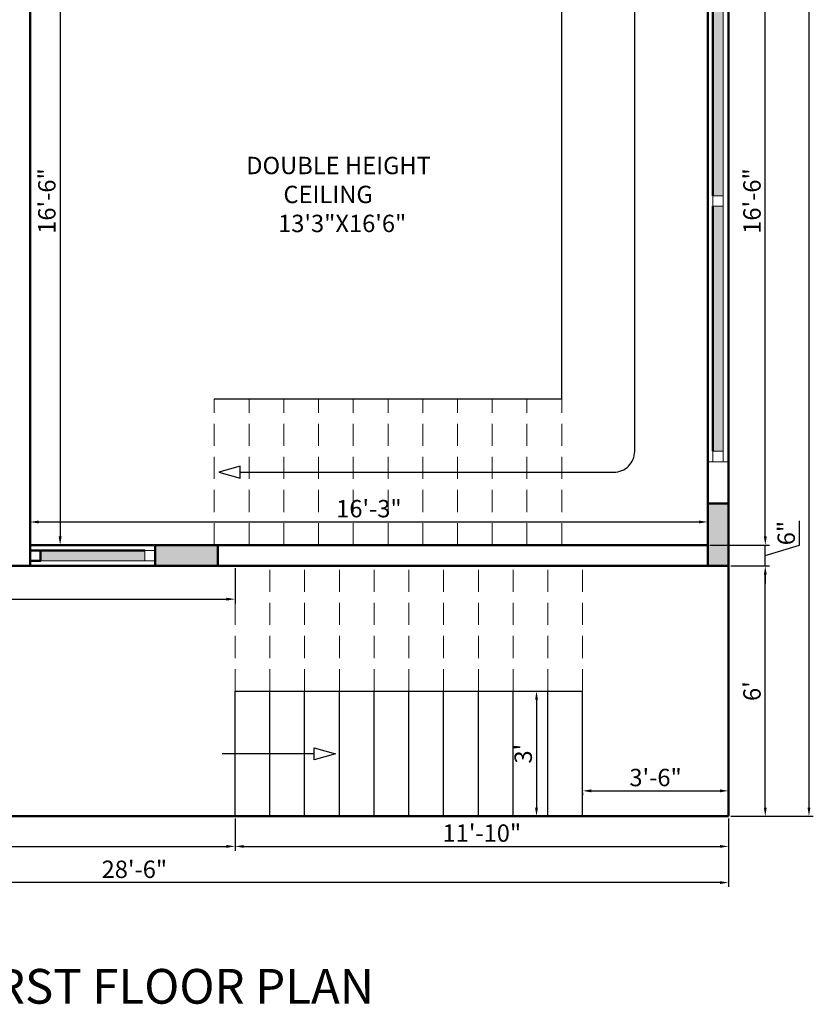
# Model space of a CAD drawing. Units: inches. Extents: x 3064 to 19385, y 846 to 15425.
# Tile 99 of 108: x 7664 to 7893, y 850 to 1134. Entities that reach past the tile are written whole.
import ezdxf

# ---------------------------------------------------------------- set-up
doc = ezdxf.new("R2010")
doc.units = ezdxf.units.IN
doc.linetypes.add('DASHED', pattern=[19.05, 12.7, -6.35])
for name, color, linetype, lineweight in [('A-ANNO-DIMS', 2, 'Continuous', 18), ('A-ANNO-TEXT', 7, 'Continuous', 25), ('A-AREA-IDEN', 3, 'Continuous', 18), ('A-COLS', 1, 'Continuous', 35), ('A-FLOR-STRS', 2, 'Continuous', 25), ('A-FLOR-STRS-OVHD', 2, 'DASHED', 18), ('A-GLAZ', 4, 'Continuous', 18), ('A-WALL', 7, 'Continuous', 50)]:
    doc.layers.add(name, color=color, linetype=linetype, lineweight=lineweight)
doc.styles.get("Standard").update_dxf_attribs({"font": 'arial.ttf'})
doc.dimstyles.new('ISO-25', dxfattribs={"dimtxt": 9, "dimasz": 2.5, "dimexe": 1.25, "dimexo": 0.625, "dimtad": 1, "dimdec": 1, "dimlunit": 3, "dimtxsty": 'Standard', "dimcen": 2.5, "dimadec": 0, "dimazin": 0, "dimtfac": 1, "dimtdec": 1, "dimtmove": 0, "dimatfit": 3, "dimfxl": 1, "dimarcsym": 0})

# ---------------------------------------------------------------- blocks, each defined once
blk = doc.blocks.new('*D325')
at = {"layer": 'A-ANNO-DIMS', "color": 0, "lineweight": -2, "transparency": 16777216}
for p, q in [((7526.25, 903.71), (7526.25, 894.42)), ((7726.25, 903.71), (7726.25, 894.42)), ((7528.75, 895.67), (7723.75, 895.67))]:
    blk.add_line(p, q, dxfattribs=at)
at = {"layer": 'A-ANNO-DIMS', "color": 0, "transparency": 16777216}
for points in [[(7528.75, 896.08), (7528.75, 895.25), (7526.25, 895.67)], [(7723.75, 896.08), (7723.75, 895.25), (7726.25, 895.67)]]:
    blk.add_solid(points, dxfattribs=at)
at = {"layer": 'Defpoints', "color": 0, "transparency": 16777216}
for p in [(7526.25, 904.34), (7726.25, 904.34), (7726.25, 895.67)]:
    blk.add_point(p, dxfattribs=at)
at = {"layer": 'A-ANNO-DIMS', "color": 0, "transparency": 16777216, "insert": (7626.25, 898.85), "char_height": 5, "attachment_point": 5}
blk.add_mtext('16\'-8"', dxfattribs=at)
blk = doc.blocks.new('*D326')
at = {"layer": 'A-ANNO-DIMS', "color": 0, "lineweight": -2, "transparency": 16777216}
for p, q in [((7726.25, 903.71), (7726.25, 894.42)), ((7868.25, 903.71), (7868.25, 894.42)), ((7728.75, 895.67), (7865.75, 895.67))]:
    blk.add_line(p, q, dxfattribs=at)
at = {"layer": 'A-ANNO-DIMS', "color": 0, "transparency": 16777216}
for points in [[(7728.75, 896.08), (7728.75, 895.25), (7726.25, 895.67)], [(7865.75, 896.08), (7865.75, 895.25), (7868.25, 895.67)]]:
    blk.add_solid(points, dxfattribs=at)
at = {"layer": 'Defpoints', "color": 0, "transparency": 16777216}
for p in [(7726.25, 904.34), (7868.25, 904.34), (7868.25, 895.67)]:
    blk.add_point(p, dxfattribs=at)
at = {"layer": 'A-ANNO-DIMS', "color": 0, "transparency": 16777216, "insert": (7797.25, 898.85), "char_height": 5, "attachment_point": 5}
blk.add_mtext('11\'-10"', dxfattribs=at)
blk = doc.blocks.new('*D224')
at = {"layer": 'A-ANNO-DIMS', "color": 0, "lineweight": -2, "transparency": 16777216}
for p, q in [((7526.25, 903.71), (7526.25, 884.01)), ((7868.25, 903.71), (7868.25, 884.01)), ((7865.75, 885.26), (7528.75, 885.26))]:
    blk.add_line(p, q, dxfattribs=at)
at = {"layer": 'A-ANNO-DIMS', "color": 0, "transparency": 16777216}
for points in [[(7528.75, 885.67), (7528.75, 884.84), (7526.25, 885.26)], [(7865.75, 885.67), (7865.75, 884.84), (7868.25, 885.26)]]:
    blk.add_solid(points, dxfattribs=at)
at = {"layer": 'Defpoints', "color": 0, "transparency": 16777216}
for p in [(7526.25, 904.34), (7868.25, 904.34), (7526.25, 885.26)]:
    blk.add_point(p, dxfattribs=at)
at = {"layer": 'A-ANNO-DIMS', "color": 0, "transparency": 16777216, "insert": (7697.25, 888.43), "char_height": 5, "attachment_point": 5}
blk.add_mtext('28\'-6"', dxfattribs=at)
blk = doc.blocks.new('*D327')
at = {"layer": 'A-ANNO-DIMS', "color": 0, "lineweight": -2, "transparency": 16777216}
for p, q in [((7868.87, 976.34), (7880.08, 976.34)), ((7878.83, 906.84), (7878.83, 973.84)), ((7868.87, 904.34), (7880.08, 904.34))]:
    blk.add_line(p, q, dxfattribs=at)
at = {"layer": 'A-ANNO-DIMS', "color": 0, "transparency": 16777216}
for points in [[(7878.41, 973.84), (7879.25, 973.84), (7878.83, 976.34)], [(7878.41, 906.84), (7879.25, 906.84), (7878.83, 904.34)]]:
    blk.add_solid(points, dxfattribs=at)
at = {"layer": 'Defpoints', "color": 0, "transparency": 16777216}
for p in [(7868.25, 976.34), (7878.83, 976.34), (7868.25, 904.34)]:
    blk.add_point(p, dxfattribs=at)
at = {"layer": 'A-ANNO-DIMS', "color": 0, "transparency": 16777216, "insert": (7875.65, 940.34), "char_height": 5, "attachment_point": 5, "rotation": 90}
blk.add_mtext("6'", dxfattribs=at)
blk = doc.blocks.new('*D328')
at = {"layer": 'A-ANNO-DIMS', "color": 0, "lineweight": -2, "transparency": 16777216}
for p, q in [((7888.67, 982.29), (7888.67, 989.32)), ((7878.83, 984.84), (7878.83, 987.34)), ((7862.87, 982.34), (7880.08, 982.34)), ((7878.83, 976.34), (7878.83, 982.34)), ((7878.83, 976.34), (7878.83, 982.34)), ((7878.83, 979.34), (7888.67, 982.29)), ((7868.87, 976.34), (7880.08, 976.34)), ((7878.83, 973.84), (7878.83, 971.34))]:
    blk.add_line(p, q, dxfattribs=at)
at = {"layer": 'A-ANNO-DIMS', "color": 0, "transparency": 16777216}
for points in [[(7878.41, 984.84), (7879.25, 984.84), (7878.83, 982.34)], [(7878.41, 973.84), (7879.25, 973.84), (7878.83, 976.34)]]:
    blk.add_solid(points, dxfattribs=at)
at = {"layer": 'Defpoints', "color": 0, "transparency": 16777216}
for p in [(7862.25, 982.34), (7878.83, 982.34), (7868.25, 976.34)]:
    blk.add_point(p, dxfattribs=at)
at = {"layer": 'A-ANNO-DIMS', "color": 0, "transparency": 16777216, "insert": (7885.5, 985.81), "char_height": 5, "attachment_point": 5, "rotation": 90}
blk.add_mtext('6"', dxfattribs=at)
blk = doc.blocks.new('*D329')
at = {"layer": 'A-ANNO-DIMS', "color": 0, "lineweight": -2, "transparency": 16777216}
for p, q in [((7868.87, 1180.34), (7880.08, 1180.34)), ((7878.83, 984.84), (7878.83, 1177.84)), ((7862.87, 982.34), (7880.08, 982.34))]:
    blk.add_line(p, q, dxfattribs=at)
at = {"layer": 'A-ANNO-DIMS', "color": 0, "transparency": 16777216}
for points in [[(7878.41, 1177.84), (7879.25, 1177.84), (7878.83, 1180.34)], [(7878.41, 984.84), (7879.25, 984.84), (7878.83, 982.34)]]:
    blk.add_solid(points, dxfattribs=at)
at = {"layer": 'Defpoints', "color": 0, "transparency": 16777216}
for p in [(7868.25, 1180.34), (7878.83, 1180.34), (7862.25, 982.34)]:
    blk.add_point(p, dxfattribs=at)
at = {"layer": 'A-ANNO-DIMS', "color": 0, "transparency": 16777216, "insert": (7875.65, 1081.34), "char_height": 5, "attachment_point": 5, "rotation": 90}
blk.add_mtext('16\'-6"', dxfattribs=at)
blk = doc.blocks.new('*D335')
at = {"layer": 'A-ANNO-DIMS', "color": 0, "lineweight": -2, "transparency": 16777216}
for p, q in [((7868.87, 1396.34), (7892.65, 1396.34)), ((7891.4, 1393.84), (7891.4, 906.84)), ((7868.87, 904.34), (7892.65, 904.34))]:
    blk.add_line(p, q, dxfattribs=at)
at = {"layer": 'A-ANNO-DIMS', "color": 0, "transparency": 16777216}
for points in [[(7890.98, 1393.84), (7891.82, 1393.84), (7891.4, 1396.34)], [(7890.98, 906.84), (7891.82, 906.84), (7891.4, 904.34)]]:
    blk.add_solid(points, dxfattribs=at)
at = {"layer": 'Defpoints', "color": 0, "transparency": 16777216}
for p in [(7868.25, 1396.34), (7868.25, 904.34), (7891.4, 904.34)]:
    blk.add_point(p, dxfattribs=at)
at = {"layer": 'A-ANNO-DIMS', "color": 0, "transparency": 16777216, "insert": (7888.27, 1150.34), "char_height": 5, "attachment_point": 5, "rotation": 90}
blk.add_mtext("41'", dxfattribs=at)
blk = doc.blocks.new('*D265')
at = {"layer": 'A-ANNO-DIMS', "color": 0, "lineweight": -2, "transparency": 16777216}
for p, q in [((7526.25, 975.71), (7526.25, 965.55)), ((7726.25, 975.71), (7726.25, 965.55)), ((7528.75, 966.8), (7723.75, 966.8))]:
    blk.add_line(p, q, dxfattribs=at)
at = {"layer": 'A-ANNO-DIMS', "color": 0, "transparency": 16777216}
for points in [[(7528.75, 967.22), (7528.75, 966.39), (7526.25, 966.8)], [(7723.75, 967.22), (7723.75, 966.39), (7726.25, 966.8)]]:
    blk.add_solid(points, dxfattribs=at)
at = {"layer": 'Defpoints', "color": 0, "transparency": 16777216}
for p in [(7526.25, 976.34), (7726.25, 976.34), (7726.25, 966.8)]:
    blk.add_point(p, dxfattribs=at)
at = {"layer": 'A-ANNO-DIMS', "color": 0, "transparency": 16777216, "insert": (7626.25, 969.98), "char_height": 5, "attachment_point": 5}
blk.add_mtext('16\'-8"', dxfattribs=at)
blk = doc.blocks.new('*D266')
at = {"layer": 'A-ANNO-DIMS', "color": 0, "lineweight": -2, "transparency": 16777216}
for p, q in [((7868.25, 912.28), (7868.25, 912.9)), ((7826.25, 911.03), (7826.25, 910.4)), ((7828.75, 911.65), (7865.75, 911.65))]:
    blk.add_line(p, q, dxfattribs=at)
at = {"layer": 'A-ANNO-DIMS', "color": 0, "transparency": 16777216}
for points in [[(7828.75, 912.07), (7828.75, 911.23), (7826.25, 911.65)], [(7865.75, 912.07), (7865.75, 911.23), (7868.25, 911.65)]]:
    blk.add_solid(points, dxfattribs=at)
at = {"layer": 'Defpoints', "color": 0, "transparency": 16777216}
for p in [(7826.25, 911.65), (7868.25, 911.65), (7868.25, 911.65)]:
    blk.add_point(p, dxfattribs=at)
at = {"layer": 'A-ANNO-DIMS', "color": 0, "transparency": 16777216, "insert": (7847.25, 914.83), "char_height": 5, "attachment_point": 5}
blk.add_mtext('3\'-6"', dxfattribs=at)
blk = doc.blocks.new('*D259')
at = {"layer": 'A-ANNO-DIMS', "color": 0, "lineweight": -2, "transparency": 16777216}
for p, q in [((7811.42, 940.34), (7814.24, 940.34)), ((7812.99, 937.84), (7812.99, 906.84)), ((7811.42, 904.34), (7814.24, 904.34))]:
    blk.add_line(p, q, dxfattribs=at)
at = {"layer": 'A-ANNO-DIMS', "color": 0, "transparency": 16777216}
for points in [[(7812.57, 937.84), (7813.41, 937.84), (7812.99, 940.34)], [(7812.57, 906.84), (7813.41, 906.84), (7812.99, 904.34)]]:
    blk.add_solid(points, dxfattribs=at)
at = {"layer": 'Defpoints', "color": 0, "transparency": 16777216}
for p in [(7810.8, 940.34), (7810.8, 904.34), (7812.99, 904.34)]:
    blk.add_point(p, dxfattribs=at)
at = {"layer": 'A-ANNO-DIMS', "color": 0, "transparency": 16777216, "insert": (7809.81, 922.34), "char_height": 5, "attachment_point": 5, "rotation": 90}
blk.add_mtext("3'", dxfattribs=at)
blk = doc.blocks.new('*D244')
at = {"layer": 'A-ANNO-DIMS', "color": 0, "lineweight": -2, "transparency": 16777216}
for p, q in [((7667.87, 1180.34), (7677.14, 1180.34)), ((7675.89, 1177.84), (7675.89, 984.84)), ((7667.87, 982.34), (7677.14, 982.34))]:
    blk.add_line(p, q, dxfattribs=at)
at = {"layer": 'A-ANNO-DIMS', "color": 0, "transparency": 16777216}
for points in [[(7675.47, 1177.84), (7676.3, 1177.84), (7675.89, 1180.34)], [(7675.47, 984.84), (7676.3, 984.84), (7675.89, 982.34)]]:
    blk.add_solid(points, dxfattribs=at)
at = {"layer": 'Defpoints', "color": 0, "transparency": 16777216}
for p in [(7667.25, 1180.34), (7667.25, 982.34), (7675.89, 982.34)]:
    blk.add_point(p, dxfattribs=at)
at = {"layer": 'A-ANNO-DIMS', "color": 0, "transparency": 16777216, "insert": (7672.71, 1081.34), "char_height": 5, "attachment_point": 5, "rotation": 90}
blk.add_mtext('16\'-6"', dxfattribs=at)
blk = doc.blocks.new('*D245')
at = {"layer": 'A-ANNO-DIMS', "color": 0, "lineweight": -2, "transparency": 16777216}
for p, q in [((7667.25, 982.96), (7667.25, 990.26)), ((7669.75, 989.01), (7859.75, 989.01)), ((7862.25, 982.96), (7862.25, 990.26))]:
    blk.add_line(p, q, dxfattribs=at)
at = {"layer": 'A-ANNO-DIMS', "color": 0, "transparency": 16777216}
for points in [[(7669.75, 989.43), (7669.75, 988.6), (7667.25, 989.01)], [(7859.75, 989.43), (7859.75, 988.6), (7862.25, 989.01)]]:
    blk.add_solid(points, dxfattribs=at)
at = {"layer": 'Defpoints', "color": 0, "transparency": 16777216}
for p in [(7862.25, 989.01), (7667.25, 982.34), (7862.25, 982.34)]:
    blk.add_point(p, dxfattribs=at)
at = {"layer": 'A-ANNO-DIMS', "color": 0, "transparency": 16777216, "insert": (7764.75, 992.19), "char_height": 5, "attachment_point": 5}
blk.add_mtext('16\'-3"', dxfattribs=at)
blk = doc.blocks.new('WIN-1800-PAIR')
h = blk.add_hatch(color=256)
h.dxf.hatch_style = 1
h.paths.add_polyline_path([(0, 0), (3, 0), (3, 70.5), (0, 70.5)])
h.paths.add_polyline_path([(3, 144), (0, 144), (0, 73.5), (3, 73.5)])
blk.add_line((3, 144), (3, 73.5))
blk.add_lwpolyline([(3, 144), (0, 144), (0, 147), (3, 147)], close=True)
blk = doc.blocks.new('WIN-900')
blk.add_line((0, 0), (30, 0))
blk.add_lwpolyline([(30, 0), (30, 3), (33, 3), (33, 0)], close=True)
blk = doc.blocks.new('WIN-2000')
blk.add_line((3, 0), (3, 70.5))
blk.add_lwpolyline([(3, 70.5), (0, 70.5), (0, 73.5), (3, 73.5)], close=True)

msp = doc.modelspace()

# ---------------------------------------------------------------- hatches: boundary and pattern name
at = {"layer": 'A-COLS'}
h = msp.add_hatch(color=256, dxfattribs=at)
h.dxf.hatch_style = 1
h.paths.add_polyline_path([(7862.25, 976.34), (7868.25, 976.34), (7868.25, 994.34), (7862.25, 994.34)])
h = msp.add_hatch(color=256, dxfattribs=at)
h.dxf.hatch_style = 1
h.paths.add_polyline_path([(7721.25, 976.34), (7721.25, 982.34), (7703.25, 982.34), (7703.25, 976.34)])
at = {"layer": 'A-GLAZ'}
h = msp.add_hatch(color=256, dxfattribs=at)
h.dxf.hatch_style = 1
h.paths.add_polyline_path([(7670.25, 980.84), (7670.25, 977.84), (7700.25, 977.84), (7700.25, 980.84)])

# ---------------------------------------------------------------- linework, layer by layer
at = {"layer": 'A-FLOR-STRS'}
for p, q in [((7820.25, 1024.34), (7820.25, 1180.34)), ((7820.25, 1024.34), (7720.25, 1024.34)), ((7726.25, 904.34), (7726.25, 940.34)), ((7726.25, 940.34), (7826.25, 940.34)), ((7736.25, 904.34), (7736.25, 940.34)), ((7746.25, 904.34), (7746.25, 940.34)), ((7756.25, 904.34), (7756.25, 940.34)), ((7766.25, 904.34), (7766.25, 940.34)), ((7776.25, 904.34), (7776.25, 940.34)), ((7786.25, 904.34), (7786.25, 940.34)), ((7796.25, 904.34), (7796.25, 940.34)), ((7806.25, 904.34), (7806.25, 940.34)), ((7816.25, 904.34), (7816.25, 940.34)), ((7826.25, 904.34), (7826.25, 940.34)), ((7748.95, 922.34), (7722.56, 922.34))]:
    msp.add_line(p, q, dxfattribs=at)
msp.add_lwpolyline([(7727.74, 1003.34), (7835.25, 1003.34, 0.414214), (7841.25, 1009.34), (7841.25, 1153.34, 0.414214), (7835.25, 1159.34), (7708.25, 1159.34)], format="xyb", dxfattribs=at)
for points in [[(7721.54, 1003.34), (7727.74, 1001.61), (7727.74, 1005.07)], [(7755.14, 922.34), (7748.95, 920.61), (7748.95, 924.07)]]:
    msp.add_lwpolyline(points, close=True, dxfattribs=at)
at = {"layer": 'A-FLOR-STRS-OVHD', "ltscale": 0.5}
for p, q in [((7720.25, 982.34), (7720.25, 1024.34)), ((7730.25, 982.34), (7730.25, 1024.34)), ((7740.25, 982.34), (7740.25, 1024.34)), ((7750.25, 982.34), (7750.25, 1024.34)), ((7760.25, 982.34), (7760.25, 1024.34)), ((7770.25, 982.34), (7770.25, 1024.34)), ((7780.25, 982.34), (7780.25, 1024.34)), ((7790.25, 982.34), (7790.25, 1024.34)), ((7800.25, 982.34), (7800.25, 1024.34)), ((7810.25, 982.34), (7810.25, 1024.34)), ((7820.25, 982.34), (7820.25, 1024.34)), ((7726.25, 940.34), (7726.25, 976.34)), ((7736.25, 940.34), (7736.25, 976.34)), ((7746.25, 940.34), (7746.25, 976.34)), ((7756.25, 940.34), (7756.25, 976.34)), ((7766.25, 940.34), (7766.25, 976.34)), ((7776.25, 940.34), (7776.25, 976.34)), ((7786.25, 940.34), (7786.25, 976.34)), ((7796.25, 940.34), (7796.25, 976.34)), ((7806.25, 940.34), (7806.25, 976.34)), ((7816.25, 940.34), (7816.25, 976.34)), ((7826.25, 940.34), (7826.25, 976.34))]:
    msp.add_line(p, q, dxfattribs=at)
at = {"layer": 'A-GLAZ'}
msp.add_line((7868.25, 1006.34), (7862.25, 1006.34), dxfattribs=at)
msp.add_line((7868.25, 1006.34), (7862.25, 1006.34), dxfattribs=at)
msp.add_lwpolyline([(7866.75, 1006.34), (7863.75, 1006.34), (7863.75, 1009.34), (7866.75, 1009.34)], close=True, dxfattribs=at)
at = {"layer": 'A-WALL'}
for p, q in [((7868.25, 904.34), (7868.25, 1396.34)), ((7862.25, 982.34), (7862.25, 1180.34)), ((7863.75, 1153.34), (7863.75, 1082.84)), ((7667.25, 1144.34), (7667.25, 976.34)), ((7863.75, 1009.34), (7863.75, 1079.84)), ((7862.25, 982.34), (7667.25, 982.34)), ((7667.25, 976.34), (7667.25, 982.34)), ((7670.25, 980.84), (7700.25, 980.84)), ((7703.25, 976.34), (7703.25, 982.34)), ((7703.25, 976.34), (7703.25, 982.34)), ((7868.25, 976.34), (7526.25, 976.34)), ((7526.25, 904.34), (7868.25, 904.34))]:
    msp.add_line(p, q, dxfattribs=at)
for points in [[(7868.25, 976.34), (7868.25, 994.34), (7862.25, 994.34), (7862.25, 976.34)], [(7667.25, 977.84), (7667.25, 980.84), (7670.25, 980.84), (7670.25, 977.84)], [(7721.25, 982.34), (7703.25, 982.34), (7703.25, 976.34), (7721.25, 976.34)]]:
    msp.add_lwpolyline(points, close=True, dxfattribs=at)

# ---------------------------------------------------------------- block references
at = {"layer": 'A-GLAZ'}
for name, p in [('WIN-1800-PAIR', (7863.75, 1009.34)), ('WIN-2000', (7863.75, 1009.34)), ('WIN-900', (7670.25, 977.84))]:
    msp.add_blockref(name, p, dxfattribs=at)

# ---------------------------------------------------------------- texts
at = {"layer": 'A-ANNO-TEXT', "insert": (7645.59, 860.41), "char_height": 10, "attachment_point": 1}
msp.add_mtext_dynamic_manual_height_columns('FIRST FLOOR PLAN', width=200.9739, gutter_width=12.5, heights=[0], dxfattribs=at)
at = {"layer": 'A-AREA-IDEN', "insert": (7729.45, 1094.07), "char_height": 5, "attachment_point": 1}
msp.add_mtext_dynamic_manual_height_columns('DOUBLE HEIGHT \\P       CEILING            \\P      13\'3"X16\'6"', width=57.0817, gutter_width=12.5, heights=[0], dxfattribs=at)

# ---------------------------------------------------------------- dimensions: what is measured, and where the dimension line sits
at = {"layer": 'A-ANNO-DIMS'}
for base, p1, p2, override, picture, middle in [((7891.4, 904.34), (7868.25, 1396.34), (7868.25, 904.34), {"dimtxt": 5, "dimclrd": 0, "dimclre": 0, "dimclrt": 0}, '*D335', (7888.27, 1150.34)), ((7675.89, 982.34), (7667.25, 1180.34), (7667.25, 982.34), {"dimtxt": 5, "dimclrd": 0, "dimclre": 0, "dimclrt": 0}, '*D244', (7672.71, 1081.34)), ((7878.83, 1180.34), (7862.25, 982.34), (7868.25, 1180.34), {"dimtxt": 5, "dimclrd": 0, "dimclre": 0, "dimclrt": 0, "dimtmove": 1}, '*D329', (7875.65, 1081.34)), ((7878.83, 982.34), (7868.25, 976.34), (7862.25, 982.34), {"dimtxt": 5, "dimclrd": 0, "dimclre": 0, "dimclrt": 0, "dimtmove": 1}, '*D328', (7885.5, 982.92)), ((7878.83, 976.34), (7868.25, 904.34), (7868.25, 976.34), {"dimtxt": 5, "dimclrd": 0, "dimclre": 0, "dimclrt": 0}, '*D327', (7875.65, 940.34)), ((7812.99, 904.34), (7810.8, 940.34), (7810.8, 904.34), {"dimtxt": 5, "dimclrd": 0, "dimclre": 0, "dimclrt": 0}, '*D259', (7809.81, 922.34))]:
    dim = msp.add_linear_dim(base=base, p1=p1, p2=p2, angle=90, dimstyle='ISO-25', override=override, dxfattribs=at)
    dim.commit()
    dim.dimension.update_dxf_attribs({"geometry": picture, "text_midpoint": middle})
for base, p1, p2, override, picture, middle in [((7862.25, 989.01), (7667.25, 982.34), (7862.25, 982.34), {"dimtxt": 5, "dimclrd": 0, "dimclre": 0, "dimclrt": 0}, '*D245', (7764.75, 992.19)), ((7726.25, 966.8), (7526.25, 976.34), (7726.25, 976.34), {"dimtxt": 5, "dimclrd": 0, "dimclre": 0, "dimclrt": 0}, '*D265', (7626.25, 969.98)), ((7868.25, 911.65), (7826.25, 911.65), (7868.25, 911.65), {"dimtxt": 5, "dimclrd": 0, "dimclre": 0, "dimclrt": 0}, '*D266', (7847.25, 914.83)), ((7726.25, 895.67), (7526.25, 904.34), (7726.25, 904.34), {"dimtxt": 5, "dimclrd": 0, "dimclre": 0, "dimclrt": 0}, '*D325', (7626.25, 898.85)), ((7526.25, 885.26), (7868.25, 904.34), (7526.25, 904.34), {"dimtxt": 5, "dimclrd": 0, "dimclre": 0, "dimclrt": 0}, '*D224', (7697.25, 888.43)), ((7868.25, 895.67), (7726.25, 904.34), (7868.25, 904.34), {"dimtxt": 5, "dimclrd": 0, "dimclre": 0, "dimclrt": 0, "dimtmove": 1}, '*D326', (7797.25, 898.85))]:
    dim = msp.add_linear_dim(base=base, p1=p1, p2=p2, dimstyle='ISO-25', override=override, dxfattribs=at)
    dim.commit()
    dim.dimension.update_dxf_attribs({"geometry": picture, "text_midpoint": middle})

doc.saveas('drawing.dxf')
